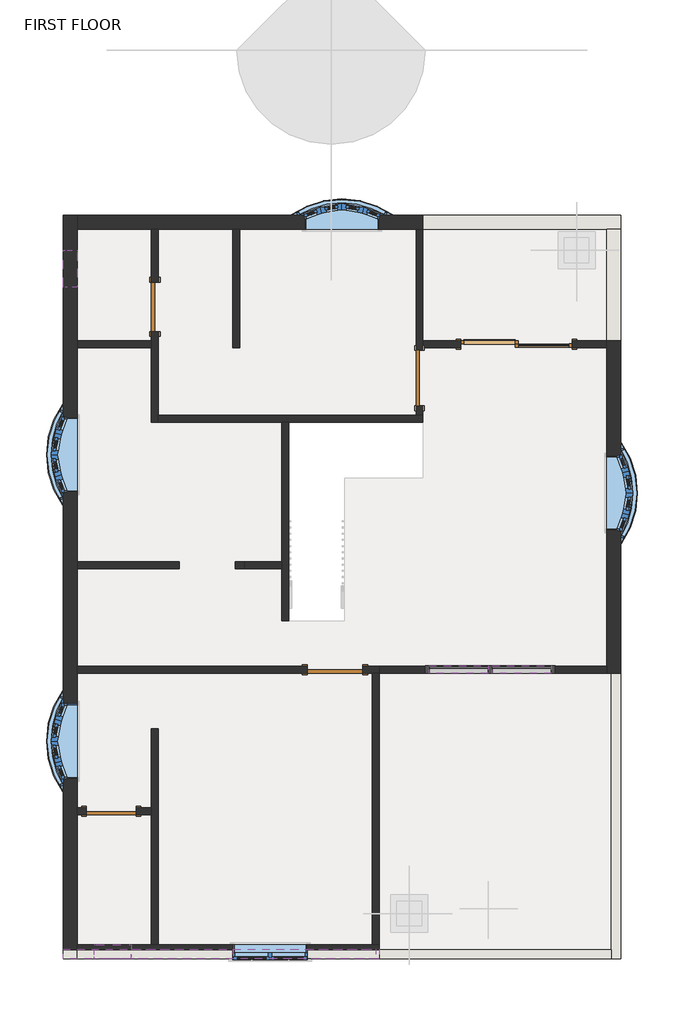
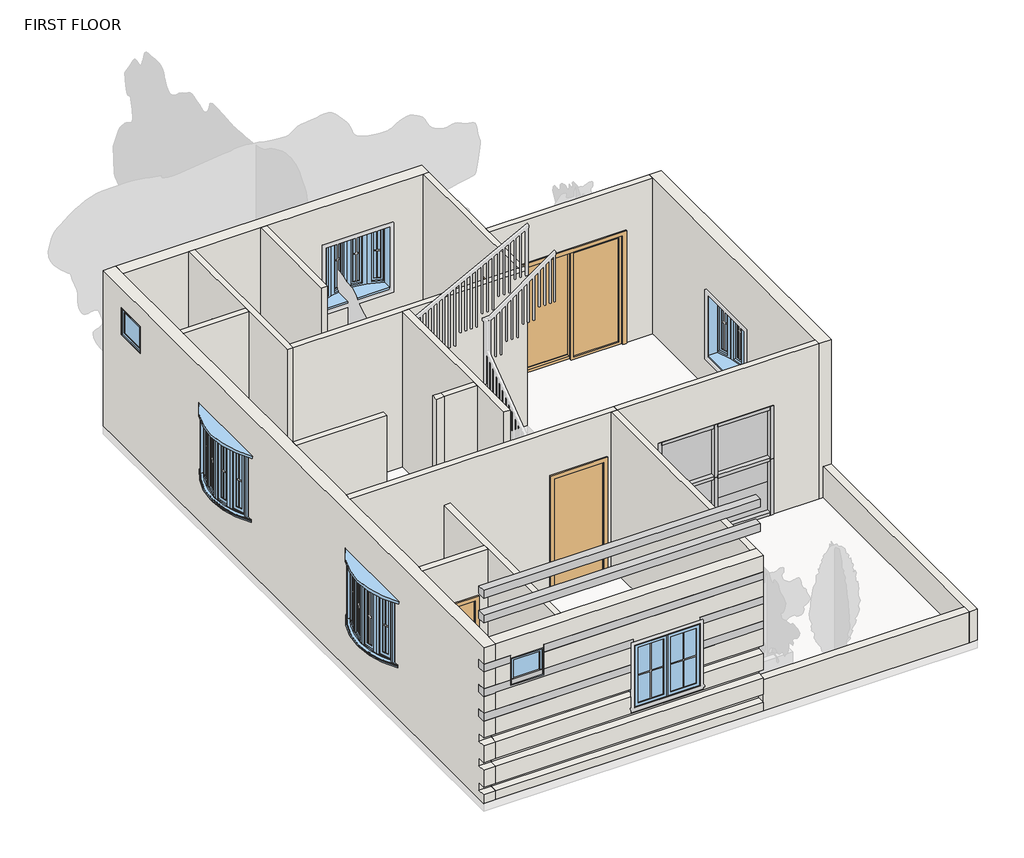
# One storey, part 1 of 2: 23 walls, 12 members, 7 windows, 5 doors, 5 plates, 5 proxies.
# Revit data of these elements (continued)
# Elements 45, 46 (IfcWall, "9\"") (continued)
#   Base Constraint = FIRST FLOOR
#   Top Constraint = SECOND FLOOR
#   Materials on its faces: "wood", "wall 2"
# Elements 47, 48 (IfcWall, "9\"")
#   Top Offset = -0' - 6"
#   Base Offset = 0' - 0"
#   wall height = 10' - 0"
#   Phase Created = New Construction
#   Base Constraint = FIRST FLOOR
#   Top Constraint = SECOND FLOOR
#   Materials on its faces: "wood", "wall 2", "wall 1"
# Element 49 (IfcWall, "9\"")
#   Top Offset = -0' - 6"
#   Base Offset = 0' - 0"
#   Unconnected Height = 2' - 0"
#   wall height = 2' - 0"
#   Phase Created = New Construction
#   Base Constraint = FIRST FLOOR
#   Materials on its faces: "wall 1", "wood", "6\" wall"
# Element 50 (IfcWall, "9\"")
#   Top Offset = -0' - 6"
#   Base Offset = 0' - 0"
#   Unconnected Height = 2' - 0"
#   wall height = 2' - 0"
#   Phase Created = New Construction
#   Base Constraint = FIRST FLOOR
#   Materials on its faces: "wood", "wall 1"
# Element 51 (IfcWindow, "Fixed : 2'X1'9\"")
#   Mark = "13"
#   Phase Created = New Construction
#   Materials on its faces: "Sash", "Glass"
# Element 52 (IfcWindow, "Fixed : 2'X1'9\"")
#   Mark = "14"
#   Phase Created = New Construction
#   Materials on its faces: "Sash", "Glass"
# Element 53 (IfcWindow, "Window-Bow-Casement-10_Degree_Angle : 4'X4'")
#   Mark = "9"
#   Phase Created = New Construction
#   Materials on its faces: "Wood - Stained", "Clad - White", "Glass"
# Element 54 (IfcWindow, "Window-Bow-Casement-10_Degree_Angle : 4'X4'")
#   Mark = "10"
#   Phase Created = New Construction
#   Materials on its faces: "Wood - Stained", "Clad - White", "Glass"
# Element 55 (IfcWindow, "Window-Bow-Casement-10_Degree_Angle : 4'X4'")
#   Mark = "11"
#   Phase Created = New Construction
#   Materials on its faces: "Wood - Stained", "Clad - White", "Glass"
# Element 56 (IfcWindow, "Window-Bow-Casement-10_Degree_Angle : 4'X4'")
#   Mark = "16"
#   Interior Trim Visibility = yes
#   Exterior Trim Visibility = yes
#   Phase Created = New Construction
#   Materials on its faces: "Wood - Stained", "Clad - White", "Glass"
# Element 57 (IfcWindow, "Window-Casement-Double : 4'X4'")
#   Mark = "8"
#   Window Inset = 0' - 0"
#   Interior Wall Closure = 0' - 2 1/4"
#   Frame Extension = 0' - 0 1/4"
#   Exterior Wall Closure = 0' - 1 1/4"
#   Interior Trim Visibility = yes
#   Exterior Trim Visibility = yes
#   Phase Created = New Construction
#   Materials on its faces: "Wood - Stained", "Glass", "Clad - White"
# Materials
#   "Glass": class "Glass", colour RGB 0 128 192, transparency 0.75, Description = "Soda Lime Glass", Cost = 0
#   "Wood - Birch - Solid Stained Light Low Gloss": class "Wood", colour RGB 210 159 95, transparency 0, Cost = 0
#   "Paint - Sienna": colour RGB 118 70 51, transparency 0, Cost = 0
#   "Door - Panel": class "Wood", colour RGB 210 159 95, transparency 0, Cost = 0
#   "Door - Frame": colour RGB 118 70 51, transparency 0, Cost = 0
#   "6\" wall": class "Generic", colour RGB 177 162 144, transparency 0, Cost = 0
#   "wood": class "Generic", colour RGB 188 176 153, transparency 0, Cost = 0
#   "Sash": class "Wood", colour RGB 224 178 126, transparency 0, Cost = 0
#   "Wood - Stained": class "Wood", colour RGB 224 178 126, transparency 0, Cost = 0
#   "Clad - White": class "Wood", colour RGB 242 242 238, transparency 0, Cost = 0
#   "Aluminum": class "Metal", colour RGB 247 247 247, transparency 0, Description = "Aluminum 6061", Cost = 0
#   "Default Wall": colour RGB 128 128 128, transparency 0, Cost = 0
#   "wall 1": class "Generic", colour RGB 67 39 34, transparency 0, Cost = 0
#   "wall 2": class "Generic", colour RGB 66 64 54, transparency 0, Cost = 0
